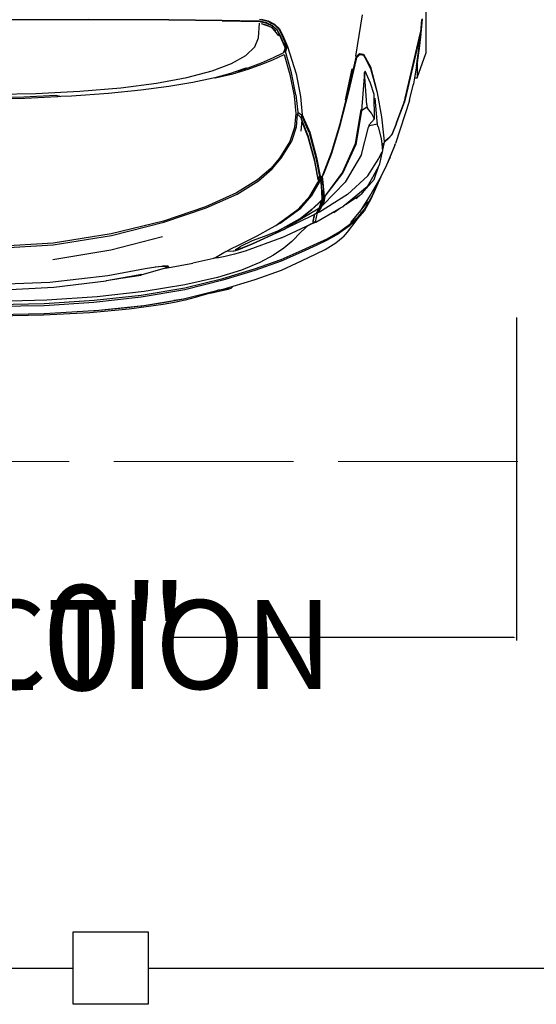
# Model space of a CAD drawing. Units: inches. Extents: x 0 to 4258, y 0 to 3769.
# Tile 7 of 30: x 3762 to 3797, y 2937 to 3003. Entities that reach past the tile are written whole.
import ezdxf

# ---------------------------------------------------------------- set-up
doc = ezdxf.new("R2010")
doc.units = ezdxf.units.IN
doc.header["$MEASUREMENT"] = 0
doc.linetypes.add('ACAD_ISO02W100', pattern=[15, 12, -3])
doc.layers.get('0').update_dxf_attribs({"color": 16})
for name, color, linetype, lineweight in [('A-ANNO-DIMS', 250, 'Continuous', 18), ('A-ANNO-TEXT', 250, 'Continuous', 18), ('A-FLOR-OVHD', 150, 'ACAD_ISO02W100', 13), ('C-PKNG-VEHI', 8, 'Continuous', 18), ('C-PROP', 150, 'Continuous', 25)]:
    doc.layers.add(name, color=color, linetype=linetype, lineweight=lineweight)
doc.layers.add('Edges', color=250, linetype='Continuous')
doc.styles.get("Standard").update_dxf_attribs({"font": 'arial.ttf'})
doc.dimstyles.get("Standard").update_dxf_attribs({"dimtxt": 7, "dimasz": 0.18, "dimexe": 0.18, "dimexo": 0.0625, "dimgap": 0.09, "dimtad": 0, "dimtih": 1, "dimtoh": 1, "dimzin": 0, "dimdsep": 46, "dimlunit": 3, "dimtxsty": 'Standard', "dimcen": 0.09, "dimadec": 0, "dimazin": 0, "dimtfac": 1, "dimtofl": 0, "dimtmove": 0, "dimatfit": 3, "dimfxl": 1, "dimtolj": 1, "dimtzin": 0, "dimarcsym": 0})

# ---------------------------------------------------------------- blocks, each defined once
blk = doc.blocks.new('Nissan Qashqai pl')
at = {"layer": 'Edges'}
for p, q in [((10.9577, 12.8101), (11.1283, 12.8101)), ((11.1783, 12.7921), (11.1283, 12.8101)), ((11.0576, 12.8026), (11.0798, 12.8008)), ((11.0768, 12.8008), (11.059, 12.8023)), ((11.0811, 12.8004), (11.0768, 12.8008)), ((11.0798, 12.8008), (11.0872, 12.7999)), ((11.0827, 12.8001), (11.0811, 12.8004)), ((11.0827, 12.8001), (11.0813, 12.7998)), ((11.0836, 12.8002), (11.0827, 12.8001)), ((11.0856, 12.7994), (11.0827, 12.8001)), ((11.0872, 12.7999), (11.0836, 12.8002)), ((11.0836, 12.8002), (11.0882, 12.7992)), ((11.2196, 12.7681), (11.0856, 12.7994)), ((11.0883, 12.7998), (11.0872, 12.7999)), ((11.0882, 12.7992), (11.2222, 12.7676)), ((11.0883, 12.7998), (11.1123, 12.797)), ((11.1147, 12.7965), (11.0883, 12.7998)), ((11.1123, 12.797), (11.1475, 12.7921)), ((11.1547, 12.791), (11.1147, 12.7965)), ((11.1475, 12.7921), (11.1525, 12.7914)), ((11.1475, 12.7921), (11.1783, 12.7921)), ((11.1525, 12.7914), (11.1547, 12.791)), ((11.1547, 12.791), (11.1783, 12.787)), ((11.1783, 12.787), (11.1783, 12.7921)), ((11.1783, 12.787), (11.1906, 12.7849)), ((11.1906, 12.7849), (11.1909, 12.7849)), ((11.193, 12.7845), (11.1909, 12.7849)), ((11.2215, 12.7775), (11.193, 12.7845)), ((11.2247, 12.7764), (11.2215, 12.7775)), ((11.2247, 12.7764), (11.3124, 12.7479)), ((11.2247, 12.767), (11.2163, 12.7689)), ((11.22, 12.768), (11.2196, 12.7681)), ((11.2247, 12.767), (11.22, 12.768)), ((11.2222, 12.7676), (11.2271, 12.7664)), ((11.2253, 12.7668), (11.2247, 12.767)), ((11.2304, 12.7649), (11.2253, 12.7668)), ((11.2253, 12.7668), (11.2271, 12.7664)), ((11.2271, 12.7664), (11.2296, 12.7658)), ((11.2271, 12.7664), (11.2277, 12.7662)), ((11.2277, 12.7662), (11.2296, 12.7658)), ((11.2732, 12.7496), (11.2277, 12.7662)), ((11.2704, 12.7504), (11.2304, 12.7649)), ((11.2702, 12.7507), (11.2704, 12.7504)), ((11.2704, 12.7506), (11.2707, 12.7503)), ((11.2707, 12.7503), (11.2704, 12.7504)), ((11.2719, 12.7498), (11.2707, 12.7503)), ((11.2934, 12.741), (11.2719, 12.7498)), ((11.2732, 12.7496), (11.2946, 12.7409)), ((11.3, 12.735), (11.2934, 12.741)), ((11.2946, 12.7409), (11.3018, 12.7346)), ((11.3081, 12.7253), (11.3, 12.735)), ((11.3018, 12.7346), (11.3103, 12.7249)), ((11.3161, 12.7467), (11.3124, 12.7479)), ((11.3161, 12.7467), (11.3376, 12.7381)), ((11.3192, 12.7454), (11.3566, 12.7294)), ((11.3405, 12.7369), (11.3376, 12.7381)), ((11.3405, 12.7369), (11.3566, 12.7294)), ((11.3566, 12.7294), (11.3796, 12.7187)), ((11.156, 12.6966), (11.203, 12.7093)), ((11.1589, 12.6971), (11.2062, 12.7098)), ((11.203, 12.7093), (11.2091, 12.7103)), ((11.2062, 12.7098), (11.2091, 12.7103)), ((11.2091, 12.7103), (11.2583, 12.7196)), ((11.2199, 12.706), (11.2666, 12.7097)), ((11.2583, 12.7196), (11.2956, 12.7234)), ((11.2666, 12.7097), (11.2729, 12.7104)), ((11.2787, 12.7123), (11.2729, 12.7104)), ((11.2729, 12.7104), (11.2766, 12.6957)), ((11.2787, 12.7123), (11.3022, 12.7186)), ((11.2956, 12.7234), (11.3085, 12.7247)), ((11.3022, 12.7186), (11.3252, 12.7213)), ((11.3086, 12.7247), (11.3081, 12.7253)), ((11.3081, 12.7253), (11.3087, 12.7247)), ((11.3085, 12.7247), (11.3086, 12.7247)), ((11.3086, 12.7247), (11.3087, 12.7247)), ((11.3087, 12.7247), (11.3103, 12.7249)), ((11.3103, 12.7249), (11.3103, 12.7249)), ((11.3103, 12.7249), (11.3106, 12.7249)), ((11.3106, 12.7249), (11.314, 12.7238)), ((11.317, 12.7227), (11.3119, 12.7236)), ((11.3132, 12.7243), (11.3256, 12.7215)), ((11.314, 12.7238), (11.317, 12.7227)), ((11.314, 12.7238), (11.3242, 12.7216)), ((11.3242, 12.7216), (11.317, 12.7227)), ((11.3198, 12.7211), (11.3252, 12.7213)), ((11.3242, 12.7216), (11.3256, 12.7215)), ((11.3252, 12.7213), (11.3283, 12.7214)), ((11.3256, 12.7215), (11.3283, 12.7214)), ((11.3283, 12.7214), (11.3297, 12.7206)), ((11.3297, 12.7206), (11.3446, 12.7173)), ((11.3297, 12.7206), (11.3302, 12.7203)), ((11.3302, 12.7203), (11.3446, 12.7173)), ((11.3302, 12.7203), (11.3394, 12.7152)), ((11.3394, 12.7152), (11.3434, 12.7138)), ((11.3394, 12.7152), (11.342, 12.7137)), ((11.379, 12.6915), (11.3434, 12.7138)), ((11.3446, 12.7173), (11.3571, 12.7146)), ((11.3583, 12.7142), (11.3571, 12.7146)), ((11.3571, 12.7146), (11.3821, 12.7008)), ((11.3583, 12.7142), (11.3821, 12.7008)), ((11.3864, 12.7044), (11.3583, 12.7142)), ((11.3796, 12.7187), (11.4164, 12.6974)), ((11.3796, 12.7187), (11.3807, 12.7182)), ((11.3807, 12.7182), (11.4267, 12.6979)), ((11.4228, 12.6989), (11.3807, 12.7182)), ((11.1298, 12.6823), (11.156, 12.6966)), ((11.1365, 12.6851), (11.1589, 12.6971)), ((11.189, 12.6968), (11.1644, 12.6862)), ((11.2337, 12.6892), (11.1672, 12.6844)), ((11.2121, 12.7043), (11.189, 12.6968)), ((11.2622, 12.7051), (11.2121, 12.7043)), ((11.2337, 12.6892), (11.2382, 12.6892)), ((11.2382, 12.6892), (11.2401, 12.6908)), ((11.2382, 12.6892), (11.2459, 12.6785)), ((11.2505, 12.6987), (11.2401, 12.6908)), ((11.2601, 12.7037), (11.2505, 12.6987)), ((11.2622, 12.7051), (11.2601, 12.7037)), ((11.2743, 12.6942), (11.2622, 12.7051)), ((11.2743, 12.6942), (11.2791, 12.6927)), ((11.335, 12.6786), (11.2791, 12.6927)), ((11.379, 12.6915), (11.417, 12.6499)), ((11.3821, 12.7008), (11.4014, 12.69)), ((11.4163, 12.6775), (11.3864, 12.7044)), ((11.4014, 12.69), (11.4022, 12.6894)), ((11.4014, 12.69), (11.4265, 12.6594)), ((11.4022, 12.6894), (11.4163, 12.6775)), ((11.4022, 12.6894), (11.4265, 12.6594)), ((11.4164, 12.6974), (11.4531, 12.6744)), ((11.4243, 12.6982), (11.4228, 12.6989)), ((11.4464, 12.6853), (11.4243, 12.6982)), ((11.4267, 12.6979), (11.4498, 12.6844)), ((11.4531, 12.6744), (11.4314, 12.6911)), ((11.1336, 12.667), (11.0492, 12.6807)), ((11.1285, 12.6745), (11.1298, 12.6823)), ((11.1293, 12.6736), (11.1285, 12.6745)), ((11.1306, 12.6812), (11.1293, 12.6736)), ((11.1353, 12.6677), (11.1293, 12.6736)), ((11.1306, 12.6752), (11.1319, 12.6827)), ((11.1319, 12.6827), (11.1306, 12.6812)), ((11.1347, 12.671), (11.1306, 12.6752)), ((11.1319, 12.6827), (11.1365, 12.6851)), ((11.1366, 12.6691), (11.1347, 12.671)), ((11.1358, 12.6676), (11.1366, 12.6691)), ((11.1401, 12.6682), (11.1366, 12.6691)), ((11.1644, 12.6862), (11.1672, 12.6844)), ((11.1672, 12.6844), (11.2459, 12.6785)), ((11.2428, 12.6769), (11.3132, 12.6652)), ((11.2459, 12.6785), (11.3153, 12.6672)), ((11.335, 12.6786), (11.3915, 12.6453)), ((11.4366, 12.6471), (11.4163, 12.6775)), ((11.4163, 12.6775), (11.4259, 12.6674)), ((11.4624, 12.6717), (11.4464, 12.6853)), ((11.4498, 12.6844), (11.4662, 12.6706)), ((11.4681, 12.6691), (11.4498, 12.6844)), ((11.4742, 12.6567), (11.4531, 12.6744)), ((11.4774, 12.6543), (11.4624, 12.6717)), ((11.4662, 12.6706), (11.4815, 12.6531)), ((11.4681, 12.6691), (11.4936, 12.6491)), ((11.1358, 12.6676), (11.1353, 12.6677)), ((11.148, 12.665), (11.1358, 12.6676)), ((11.2066, 12.6527), (11.1401, 12.6682)), ((11.2063, 12.6515), (11.148, 12.665)), ((11.2232, 12.6458), (11.1598, 12.6594)), ((11.272, 12.6349), (11.2063, 12.6515)), ((11.2728, 12.6357), (11.2066, 12.6527)), ((11.3132, 12.6652), (11.3715, 12.6398)), ((11.3733, 12.6404), (11.3153, 12.6672)), ((11.417, 12.6499), (11.4529, 12.5922)), ((11.4265, 12.6594), (11.4366, 12.6471)), ((11.4924, 12.6339), (11.4774, 12.6543)), ((11.4815, 12.6531), (11.4963, 12.6328)), ((11.4936, 12.6491), (11.5033, 12.6408)), ((11.3311, 12.6172), (11.272, 12.6349)), ((11.3323, 12.6178), (11.2728, 12.6357)), ((11.3715, 12.6398), (11.4177, 12.6052)), ((11.4203, 12.6044), (11.3733, 12.6404)), ((11.3915, 12.6453), (11.4381, 12.6002)), ((11.4366, 12.6471), (11.4408, 12.6419)), ((11.4408, 12.6419), (11.4411, 12.6414)), ((11.4411, 12.6414), (11.4411, 12.6414)), ((11.4414, 12.6409), (11.4411, 12.6414)), ((11.4414, 12.6409), (11.447, 12.6315)), ((11.4455, 12.6336), (11.4414, 12.6409)), ((11.447, 12.6315), (11.4455, 12.6336)), ((11.4455, 12.6336), (11.4462, 12.6324)), ((11.447, 12.6315), (11.4462, 12.6324)), ((11.4732, 12.585), (11.4462, 12.6324)), ((11.447, 12.6315), (11.447, 12.6314)), ((11.4536, 12.6215), (11.447, 12.6314)), ((11.5074, 12.608), (11.4924, 12.6339)), ((11.4964, 12.6326), (11.4963, 12.6328)), ((11.4964, 12.6326), (11.5113, 12.6069)), ((11.5158, 12.6256), (11.5033, 12.6408)), ((11.3751, 12.5999), (11.3311, 12.6172)), ((11.3747, 12.6011), (11.3323, 12.6178)), ((11.5165, 12.5882), (11.5074, 12.608)), ((11.5295, 12.6041), (11.5158, 12.6256)), ((11.3411, 12.5863), (11.3795, 12.5939)), ((11.3419, 12.585), (11.3804, 12.5926)), ((11.3847, 12.5899), (11.3474, 12.5827)), ((11.3863, 12.5898), (11.3493, 12.5828)), ((11.38, 12.5988), (11.3747, 12.6011)), ((11.3751, 12.5999), (11.3762, 12.5999)), ((11.3752, 12.5998), (11.3751, 12.5999)), ((11.3763, 12.5998), (11.3752, 12.5998)), ((11.3764, 12.5993), (11.3752, 12.5998)), ((11.3792, 12.5982), (11.3764, 12.5993)), ((11.3792, 12.5982), (11.3793, 12.5979)), ((11.3792, 12.5982), (11.3804, 12.5972)), ((11.3795, 12.5939), (11.3834, 12.5947)), ((11.3853, 12.5993), (11.38, 12.5988)), ((11.3804, 12.5972), (11.4082, 12.5998)), ((11.3827, 12.5953), (11.3804, 12.5972)), ((11.3804, 12.5926), (11.3841, 12.5933)), ((11.3847, 12.5899), (11.3804, 12.5926)), ((11.3811, 12.5958), (11.3808, 12.5961)), ((11.3834, 12.5947), (11.3827, 12.5953)), ((11.3846, 12.5953), (11.3829, 12.5952)), ((11.3829, 12.5952), (11.3849, 12.5951)), ((11.388, 12.591), (11.3829, 12.5952)), ((11.3834, 12.5947), (11.3841, 12.5933)), ((11.3846, 12.5953), (11.4248, 12.5976)), ((11.3846, 12.5953), (11.3846, 12.5953)), ((11.3851, 12.5951), (11.3846, 12.5953)), ((11.3846, 12.5953), (11.3849, 12.5951)), ((11.3847, 12.5899), (11.3848, 12.5899)), ((11.388, 12.591), (11.3848, 12.5899)), ((11.3849, 12.5951), (11.3851, 12.5951)), ((11.3882, 12.5923), (11.3849, 12.5951)), ((11.3851, 12.5951), (11.3867, 12.5949)), ((11.4171, 12.5766), (11.3851, 12.5951)), ((11.4212, 12.603), (11.3853, 12.5993)), ((11.3895, 12.5912), (11.3863, 12.5898)), ((11.3867, 12.5949), (11.3915, 12.5951)), ((11.3914, 12.5926), (11.3867, 12.5949)), ((11.3886, 12.5919), (11.3872, 12.5927)), ((11.3882, 12.5923), (11.3886, 12.5919)), ((11.3886, 12.5919), (11.3895, 12.5912)), ((11.3892, 12.5916), (11.3886, 12.5919)), ((11.3923, 12.5894), (11.3895, 12.5912)), ((11.4187, 12.5768), (11.3914, 12.5926)), ((11.3915, 12.5951), (11.4266, 12.5977)), ((11.4203, 12.5724), (11.3923, 12.5894)), ((11.409, 12.5999), (11.4082, 12.5998)), ((11.4164, 12.5998), (11.4082, 12.5998)), ((11.4152, 12.6004), (11.409, 12.5999)), ((11.409, 12.5999), (11.4163, 12.5999)), ((11.4173, 12.6006), (11.4152, 12.6004)), ((11.4163, 12.5999), (11.4152, 12.6004)), ((11.4163, 12.5999), (11.4186, 12.5999)), ((11.4164, 12.5998), (11.4163, 12.5999)), ((11.4181, 12.5998), (11.4164, 12.5998)), ((11.4169, 12.5996), (11.4164, 12.5998)), ((11.4252, 12.598), (11.4169, 12.5996)), ((11.4176, 12.6007), (11.4173, 12.6006)), ((11.418, 12.6006), (11.4173, 12.6006)), ((11.4215, 12.601), (11.4176, 12.6007)), ((11.418, 12.6006), (11.4176, 12.6007)), ((11.4177, 12.6052), (11.4193, 12.6042)), ((11.4204, 12.6002), (11.418, 12.6006)), ((11.4194, 12.6), (11.418, 12.6006)), ((11.4192, 12.6045), (11.4194, 12.6042)), ((11.4194, 12.6042), (11.4193, 12.6042)), ((11.4193, 12.6042), (11.4196, 12.604)), ((11.4194, 12.6042), (11.4196, 12.604)), ((11.4196, 12.6042), (11.4194, 12.6042)), ((11.4196, 12.604), (11.4201, 12.6036)), ((11.4198, 12.6041), (11.4201, 12.6036)), ((11.4201, 12.6036), (11.4212, 12.603)), ((11.4292, 12.6024), (11.4203, 12.6044)), ((11.4229, 12.6025), (11.4203, 12.6044)), ((11.4212, 12.603), (11.4215, 12.601)), ((11.4218, 12.6028), (11.4212, 12.603)), ((11.4215, 12.601), (11.4219, 12.6009)), ((11.4222, 12.6029), (11.4218, 12.6028)), ((11.4229, 12.6025), (11.4218, 12.6028)), ((11.4219, 12.6009), (11.4222, 12.6005)), ((11.4219, 12.6009), (11.4224, 12.6008)), ((11.4224, 12.6008), (11.4226, 12.6006)), ((11.4224, 12.6008), (11.423, 12.6006)), ((11.4315, 12.6002), (11.4229, 12.6025)), ((11.423, 12.6006), (11.4229, 12.6025)), ((11.44, 12.5959), (11.423, 12.6006)), ((11.4248, 12.5976), (11.4266, 12.5977)), ((11.4266, 12.5977), (11.4252, 12.598)), ((11.4266, 12.5977), (11.4268, 12.5977)), ((11.4268, 12.5977), (11.4296, 12.5954)), ((11.4268, 12.5977), (11.4278, 12.5977)), ((11.4303, 12.5956), (11.4278, 12.5977)), ((11.4278, 12.5977), (11.43, 12.5969)), ((11.4381, 12.6002), (11.4292, 12.6024)), ((11.4296, 12.5954), (11.4469, 12.5773)), ((11.4337, 12.5962), (11.43, 12.5969)), ((11.43, 12.5969), (11.4361, 12.5948)), ((11.4479, 12.5766), (11.4303, 12.5956)), ((11.4403, 12.5978), (11.4315, 12.6002)), ((11.4397, 12.5937), (11.4337, 12.5962)), ((11.4361, 12.5948), (11.4406, 12.5932)), ((11.4381, 12.6002), (11.4403, 12.5978)), ((11.4406, 12.5932), (11.4397, 12.5937)), ((11.4403, 12.5978), (11.44, 12.5959)), ((11.44, 12.5959), (11.4457, 12.5928)), ((11.4462, 12.5947), (11.4403, 12.5978)), ((11.4406, 12.5932), (11.4442, 12.592)), ((11.4442, 12.592), (11.4497, 12.589)), ((11.4462, 12.5893), (11.4442, 12.592)), ((11.4457, 12.5928), (11.4512, 12.5893)), ((11.452, 12.591), (11.4462, 12.5947)), ((11.475, 12.5409), (11.4462, 12.5893)), ((11.4497, 12.589), (11.4498, 12.5889)), ((11.4535, 12.5876), (11.4498, 12.5889)), ((11.4498, 12.5889), (11.4549, 12.5855)), ((11.4512, 12.5893), (11.4535, 12.5876)), ((11.4539, 12.5897), (11.452, 12.591)), ((11.4529, 12.5922), (11.4542, 12.5894)), ((11.4535, 12.5876), (11.4532, 12.5882)), ((11.4535, 12.5876), (11.4542, 12.5894)), ((11.4542, 12.5894), (11.4539, 12.5897)), ((11.5113, 12.6068), (11.5113, 12.6069)), ((11.5113, 12.6068), (11.5206, 12.5869)), ((11.5306, 12.5573), (11.5165, 12.5882)), ((11.5384, 12.5859), (11.5295, 12.6041)), ((11.29, 12.5711), (11.2541, 12.5557)), ((11.2586, 12.5591), (11.2895, 12.5724)), ((11.2972, 12.5692), (11.2677, 12.5575)), ((11.2993, 12.5695), (11.2705, 12.5579)), ((11.2895, 12.5724), (11.3411, 12.5863)), ((11.29, 12.5711), (11.3419, 12.585)), ((11.3474, 12.5827), (11.2972, 12.5692)), ((11.3493, 12.5828), (11.2993, 12.5695)), ((11.3474, 12.5827), (11.3474, 12.5827)), ((11.4433, 12.5543), (11.4171, 12.5766)), ((11.4447, 12.5545), (11.4187, 12.5768)), ((11.4467, 12.5488), (11.4203, 12.5724)), ((11.4469, 12.5773), (11.4659, 12.5539)), ((11.4654, 12.5548), (11.4479, 12.5766)), ((11.4535, 12.5876), (11.4728, 12.5838)), ((11.4549, 12.5855), (11.4568, 12.5836)), ((11.4564, 12.5833), (11.4567, 12.5833)), ((11.4569, 12.583), (11.4565, 12.5831)), ((11.4568, 12.5836), (11.4571, 12.5833)), ((11.4571, 12.5833), (11.4573, 12.583)), ((11.4573, 12.583), (11.4578, 12.5822)), ((11.4704, 12.5803), (11.4573, 12.583)), ((11.4573, 12.5823), (11.4574, 12.5822)), ((11.4573, 12.5823), (11.4573, 12.5823)), ((11.4576, 12.5822), (11.4574, 12.5822)), ((11.4578, 12.5822), (11.4588, 12.5807)), ((11.4605, 12.5816), (11.4578, 12.5822)), ((11.4588, 12.5807), (11.4895, 12.5178)), ((11.4713, 12.5794), (11.4605, 12.5816)), ((11.4742, 12.5797), (11.4704, 12.5803)), ((11.4744, 12.5792), (11.4713, 12.5794)), ((11.4732, 12.585), (11.4728, 12.5838)), ((11.4728, 12.5838), (11.4742, 12.5797)), ((11.4728, 12.5838), (11.4746, 12.5796)), ((11.4758, 12.5791), (11.4732, 12.585)), ((11.4742, 12.5797), (11.4744, 12.5792)), ((11.4745, 12.5797), (11.4742, 12.5797)), ((11.4745, 12.5792), (11.4744, 12.5792)), ((11.4745, 12.5792), (11.4745, 12.5797)), ((11.4745, 12.5797), (11.4746, 12.5796)), ((11.4748, 12.5792), (11.4745, 12.5792)), ((11.4746, 12.5796), (11.4748, 12.5792)), ((11.4746, 12.5796), (11.4758, 12.5791)), ((11.4758, 12.5791), (11.4748, 12.5792)), ((11.4758, 12.5791), (11.4759, 12.579)), ((11.4759, 12.579), (11.4778, 12.5746)), ((11.4759, 12.579), (11.4771, 12.576)), ((11.5057, 12.5145), (11.4771, 12.576)), ((11.4778, 12.5746), (11.4826, 12.5669)), ((11.5206, 12.5869), (11.5349, 12.5559)), ((11.5527, 12.5559), (11.5384, 12.5859)), ((11.1702, 12.5444), (11.2166, 12.5534)), ((11.2127, 12.5443), (11.2488, 12.548)), ((11.2166, 12.5534), (11.2538, 12.5571)), ((11.2488, 12.548), (11.2541, 12.5557)), ((11.2488, 12.548), (11.2524, 12.5477)), ((11.2599, 12.5552), (11.2524, 12.5477)), ((11.2785, 12.5455), (11.2524, 12.5477)), ((11.2538, 12.5571), (11.2586, 12.5591)), ((11.2541, 12.5557), (11.2599, 12.5552)), ((11.2677, 12.5575), (11.2599, 12.5552)), ((11.265, 12.5563), (11.2599, 12.5552)), ((11.2705, 12.5579), (11.265, 12.5563)), ((11.265, 12.5563), (11.2724, 12.5557)), ((11.2724, 12.5557), (11.2874, 12.5544)), ((11.4745, 12.5116), (11.4433, 12.5543)), ((11.4758, 12.5118), (11.4447, 12.5545)), ((11.4801, 12.503), (11.4467, 12.5488)), ((11.4633, 12.5594), (11.4897, 12.5108)), ((11.4654, 12.5548), (11.4659, 12.5539)), ((11.4659, 12.5539), (11.4674, 12.5512)), ((11.4675, 12.551), (11.4674, 12.5512)), ((11.4675, 12.551), (11.4703, 12.546)), ((11.4826, 12.5669), (11.4869, 12.5615)), ((11.4869, 12.5615), (11.4933, 12.555)), ((11.5131, 12.5356), (11.4933, 12.555)), ((11.5496, 12.5141), (11.5306, 12.5573)), ((11.5349, 12.5559), (11.5535, 12.5139)), ((11.5716, 12.5145), (11.5527, 12.5559)), ((11.1144, 12.5271), (11.1702, 12.5444)), ((11.1683, 12.5354), (11.1244, 12.5227)), ((11.1302, 12.52), (11.1712, 12.5317)), ((11.2127, 12.5443), (11.1683, 12.5354)), ((11.1712, 12.5317), (11.2152, 12.5404)), ((11.2152, 12.5404), (11.2509, 12.5439)), ((11.2509, 12.5439), (11.28, 12.5414)), ((11.3076, 12.5358), (11.2785, 12.5455)), ((11.28, 12.5414), (11.3082, 12.532)), ((11.3428, 12.5139), (11.3076, 12.5358)), ((11.3082, 12.532), (11.3425, 12.5106)), ((11.4703, 12.546), (11.4704, 12.5458)), ((11.4704, 12.5458), (11.4909, 12.5085)), ((11.4704, 12.5458), (11.4897, 12.5108)), ((11.475, 12.5409), (11.4828, 12.5276)), ((11.488, 12.5208), (11.4828, 12.5276)), ((11.5131, 12.5356), (11.5265, 12.5194)), ((11.0682, 12.5004), (11.0779, 12.5103)), ((11.0692, 12.4996), (11.0787, 12.5092)), ((11.0747, 12.4944), (11.092, 12.5087)), ((11.0779, 12.5103), (11.0902, 12.5166)), ((11.0787, 12.5092), (11.0908, 12.5153)), ((11.0912, 12.5117), (11.0802, 12.5057)), ((11.0917, 12.5114), (11.0809, 12.5056)), ((11.0902, 12.5166), (11.1144, 12.5271)), ((11.0908, 12.5153), (11.107, 12.5224)), ((11.1138, 12.5213), (11.0912, 12.5117)), ((11.1149, 12.5212), (11.0917, 12.5114)), ((11.107, 12.5224), (11.1116, 12.5243)), ((11.1138, 12.5213), (11.107, 12.5224)), ((11.1116, 12.5243), (11.1147, 12.5257)), ((11.1244, 12.5227), (11.1116, 12.5243)), ((11.1139, 12.5213), (11.1138, 12.5213)), ((11.1164, 12.5224), (11.1139, 12.5213)), ((11.1147, 12.5257), (11.1244, 12.5227)), ((11.1172, 12.5222), (11.1149, 12.5212)), ((11.1164, 12.5224), (11.1174, 12.5223)), ((11.1173, 12.5222), (11.1172, 12.5222)), ((11.1174, 12.5223), (11.1173, 12.5222)), ((11.12, 12.5215), (11.1174, 12.5223)), ((11.1246, 12.5199), (11.12, 12.5215)), ((11.1259, 12.5194), (11.1244, 12.5227)), ((11.1244, 12.5227), (11.126, 12.5194)), ((11.1259, 12.5194), (11.1246, 12.5199)), ((11.126, 12.5193), (11.1247, 12.5197)), ((11.126, 12.5193), (11.1248, 12.5195)), ((11.1251, 12.5189), (11.126, 12.5193)), ((11.126, 12.5193), (11.1259, 12.5194)), ((11.126, 12.5194), (11.1259, 12.5194)), ((11.126, 12.5194), (11.1261, 12.5193)), ((11.1264, 12.5192), (11.126, 12.5194)), ((11.1263, 12.5186), (11.126, 12.5193)), ((11.1261, 12.5193), (11.126, 12.5193)), ((11.1261, 12.5193), (11.1263, 12.5188)), ((11.1264, 12.5192), (11.1261, 12.5193)), ((11.1277, 12.5167), (11.1264, 12.5192)), ((11.1369, 12.4986), (11.1277, 12.5167)), ((11.1412, 12.4969), (11.1302, 12.52)), ((11.3425, 12.5106), (11.3635, 12.4929)), ((11.3645, 12.4958), (11.3428, 12.5139)), ((11.4788, 12.5052), (11.4745, 12.5116)), ((11.4852, 12.494), (11.4758, 12.5118)), ((11.5179, 12.4551), (11.488, 12.5208)), ((11.4898, 12.5172), (11.4895, 12.5178)), ((11.4897, 12.5108), (11.4909, 12.5085)), ((11.4898, 12.5172), (11.49, 12.5167)), ((11.49, 12.5167), (11.5179, 12.4551)), ((11.4909, 12.5085), (11.5028, 12.4792)), ((11.5057, 12.5145), (11.5325, 12.4404)), ((11.5265, 12.5194), (11.541, 12.4982)), ((11.5691, 12.4592), (11.5496, 12.5141)), ((11.5535, 12.5139), (11.5726, 12.46)), ((11.5908, 12.4606), (11.5716, 12.5145)), ((11.0581, 12.4738), (11.0614, 12.4872)), ((11.0614, 12.4872), (11.0682, 12.5004)), ((11.0624, 12.4866), (11.0658, 12.4932)), ((11.0658, 12.4932), (11.0692, 12.4996)), ((11.0658, 12.4932), (11.0698, 12.4925)), ((11.0698, 12.4925), (11.0659, 12.4848)), ((11.0727, 12.4966), (11.0669, 12.4849)), ((11.0671, 12.4731), (11.0747, 12.4944)), ((11.0696, 12.4836), (11.0747, 12.4944)), ((11.0718, 12.4967), (11.0698, 12.4925)), ((11.0802, 12.5057), (11.0718, 12.4967)), ((11.0809, 12.5056), (11.0727, 12.4966)), ((11.0747, 12.4944), (11.0821, 12.5029)), ((11.1475, 12.4741), (11.1369, 12.4986)), ((11.1505, 12.4742), (11.1412, 12.4969)), ((11.3635, 12.4929), (11.3872, 12.4654)), ((11.3888, 12.4678), (11.3645, 12.4958)), ((11.4801, 12.503), (11.4788, 12.5052)), ((11.4852, 12.494), (11.4801, 12.503)), ((11.5013, 12.4651), (11.4852, 12.494)), ((11.541, 12.4982), (11.5562, 12.4701)), ((11.0582, 12.47), (11.0624, 12.4866)), ((11.0618, 12.3933), (11.0632, 12.47)), ((11.0622, 12.4697), (11.0621, 12.4657)), ((11.063, 12.4728), (11.0622, 12.4697)), ((11.0659, 12.4848), (11.063, 12.4728)), ((11.0641, 12.4733), (11.0632, 12.47)), ((11.0669, 12.4849), (11.0641, 12.4733)), ((11.0962, 12.4675), (11.0662, 12.4698)), ((11.0671, 12.4731), (11.0696, 12.4836)), ((11.1148, 12.4598), (11.0962, 12.4675)), ((11.1577, 12.4465), (11.1475, 12.4741)), ((11.1605, 12.4465), (11.1505, 12.4742)), ((11.4159, 12.4242), (11.3888, 12.4678)), ((11.5028, 12.4792), (11.5118, 12.4548)), ((11.5562, 12.4701), (11.5715, 12.4326)), ((11.0621, 12.4657), (11.0607, 12.3933)), ((11.1323, 12.4415), (11.1148, 12.4598)), ((11.3872, 12.4654), (11.4138, 12.4223)), ((11.5202, 12.427), (11.5013, 12.4651)), ((11.5118, 12.4548), (11.523, 12.4311)), ((11.5118, 12.4548), (11.513, 12.4514)), ((11.5292, 12.4272), (11.5179, 12.4551)), ((11.5179, 12.4551), (11.5285, 12.4279)), ((11.5884, 12.3943), (11.5691, 12.4592)), ((11.5726, 12.46), (11.5922, 12.3947)), ((11.6042, 12.4156), (11.5908, 12.4606)), ((11.1487, 12.4126), (11.1323, 12.4415)), ((11.1643, 12.425), (11.1576, 12.4459)), ((11.1643, 12.425), (11.1577, 12.4465)), ((11.1582, 12.4416), (11.1668, 12.4177)), ((11.1583, 12.4423), (11.1643, 12.425)), ((11.1699, 12.4153), (11.1605, 12.4465)), ((11.5283, 12.4109), (11.5202, 12.427)), ((11.5301, 12.4198), (11.523, 12.4311)), ((11.5285, 12.4279), (11.5302, 12.4209)), ((11.5331, 12.4157), (11.5292, 12.4272)), ((11.5325, 12.4404), (11.5386, 12.4187)), ((11.5715, 12.4326), (11.5866, 12.3835)), ((11.164, 12.373), (11.1487, 12.4126)), ((11.1643, 12.425), (11.1668, 12.4177)), ((11.1668, 12.4177), (11.1694, 12.4104)), ((11.1694, 12.4104), (11.1781, 12.3782)), ((11.178, 12.379), (11.1699, 12.4153)), ((11.4138, 12.4223), (11.4422, 12.3594)), ((11.4445, 12.3608), (11.4159, 12.4242)), ((11.5334, 12.4014), (11.5283, 12.4109)), ((11.5302, 12.4209), (11.5301, 12.4198)), ((11.5331, 12.4157), (11.5335, 12.401)), ((11.5386, 12.4187), (11.5434, 12.3997)), ((11.6042, 12.4156), (11.6077, 12.4125)), ((11.6103, 12.395), (11.6042, 12.4156)), ((11.6077, 12.4125), (11.6094, 12.4107)), ((11.6094, 12.4107), (11.6101, 12.4085)), ((11.6101, 12.4085), (11.6127, 12.3852)), ((11.6185, 12.3689), (11.6101, 12.4085)), ((11.0607, 12.3933), (11.0595, 12.2842)), ((11.0618, 12.3933), (11.0606, 12.2841)), ((11.5326, 12.4045), (11.5333, 12.4019)), ((11.5333, 12.4019), (11.5334, 12.4014)), ((11.5335, 12.401), (11.5334, 12.4014)), ((11.5357, 12.3968), (11.5335, 12.401)), ((11.5416, 12.3863), (11.5357, 12.3968)), ((11.5434, 12.3997), (11.5461, 12.3854)), ((11.6076, 12.3166), (11.5884, 12.3943)), ((11.5922, 12.3947), (11.6118, 12.3165)), ((11.6127, 12.3852), (11.6103, 12.395)), ((11.1776, 12.3211), (11.164, 12.373)), ((11.1781, 12.3782), (11.178, 12.379)), ((11.1781, 12.3782), (11.1791, 12.3746)), ((11.1791, 12.3746), (11.1877, 12.333)), ((11.5455, 12.3793), (11.5416, 12.3863)), ((11.5472, 12.3757), (11.5455, 12.3793)), ((11.5461, 12.3854), (11.5467, 12.3822)), ((11.5467, 12.3822), (11.5571, 12.3331)), ((11.5866, 12.3835), (11.6016, 12.3166)), ((11.6127, 12.3852), (11.6174, 12.3722)), ((11.6297, 12.3166), (11.6127, 12.3852)), ((11.6174, 12.3722), (11.6185, 12.3689)), ((11.6185, 12.3689), (11.6224, 12.3567)), ((11.4422, 12.3594), (11.4712, 12.2729)), ((11.4738, 12.274), (11.4445, 12.3608)), ((11.6224, 12.3567), (11.6277, 12.3379)), ((11.1877, 12.333), (11.1958, 12.2844)), ((11.5668, 12.2816), (11.5571, 12.3331)), ((11.6277, 12.3379), (11.6328, 12.3174)), ((11.1891, 12.2586), (11.1776, 12.3211)), ((11.6016, 12.3166), (11.615, 12.2333)), ((11.6229, 12.2274), (11.6076, 12.3166)), ((11.6118, 12.3165), (11.6272, 12.2272)), ((11.6301, 12.3141), (11.6297, 12.3166)), ((11.6377, 12.2734), (11.6301, 12.3141)), ((11.6332, 12.2951), (11.6301, 12.3141)), ((11.6328, 12.3174), (11.6375, 12.2956)), ((11.6334, 12.2946), (11.6332, 12.2951)), ((11.6443, 12.2288), (11.6334, 12.2946)), ((11.6375, 12.2956), (11.6422, 12.2725)), ((11.0595, 12.2842), (11.0586, 12.1198)), ((11.0606, 12.2841), (11.0597, 12.1196)), ((11.1958, 12.2844), (11.2033, 12.2269)), ((11.4712, 12.2729), (11.4976, 12.1662)), ((11.5005, 12.167), (11.4738, 12.274)), ((11.5033, 12.271), (11.5307, 12.165)), ((11.5626, 12.2771), (11.5627, 12.2817)), ((11.5627, 12.2746), (11.5626, 12.2771)), ((11.5626, 12.2745), (11.5627, 12.2746)), ((11.5627, 12.2817), (11.5634, 12.2829)), ((11.5627, 12.2817), (11.5633, 12.2814)), ((11.5628, 12.2721), (11.5627, 12.2746)), ((11.5632, 12.2783), (11.5633, 12.2814)), ((11.5636, 12.2706), (11.5632, 12.2783)), ((11.5633, 12.2814), (11.5634, 12.2829)), ((11.5633, 12.2814), (11.5661, 12.2803)), ((11.5634, 12.2829), (11.5668, 12.2816)), ((11.565, 12.2577), (11.5636, 12.2706)), ((11.5639, 12.2809), (11.5637, 12.2764)), ((11.5637, 12.2763), (11.5637, 12.2764)), ((11.5637, 12.2764), (11.5638, 12.2762)), ((11.5638, 12.2762), (11.5641, 12.2688)), ((11.5643, 12.2808), (11.5639, 12.2809)), ((11.5641, 12.2688), (11.5656, 12.2559)), ((11.5642, 12.2771), (11.5646, 12.2778)), ((11.566, 12.2801), (11.5643, 12.2808)), ((11.5647, 12.278), (11.5649, 12.2783)), ((11.566, 12.2846), (11.5668, 12.2816)), ((11.566, 12.2801), (11.5661, 12.2803)), ((11.5662, 12.28), (11.566, 12.2801)), ((11.5661, 12.2803), (11.5662, 12.28)), ((11.5662, 12.28), (11.5661, 12.2803)), ((11.5669, 12.2797), (11.5661, 12.2803)), ((11.5669, 12.2797), (11.5662, 12.28)), ((11.5662, 12.28), (11.5662, 12.28)), ((11.5667, 12.2813), (11.567, 12.2796)), ((11.5668, 12.2816), (11.5672, 12.2796)), ((11.567, 12.2796), (11.5669, 12.2797)), ((11.5672, 12.2796), (11.567, 12.2796)), ((11.5678, 12.2766), (11.5672, 12.2796)), ((11.5673, 12.2784), (11.5677, 12.2767)), ((11.5678, 12.2766), (11.5818, 12.227)), ((11.5682, 12.2743), (11.5682, 12.2742)), ((11.5683, 12.2739), (11.5683, 12.2739)), ((11.5683, 12.2738), (11.5683, 12.2737)), ((11.6378, 12.2728), (11.6377, 12.2734)), ((11.6381, 12.2716), (11.6378, 12.2728)), ((11.639, 12.2645), (11.6378, 12.2728)), ((11.639, 12.2645), (11.6381, 12.2716)), ((11.6422, 12.2725), (11.6514, 12.2026)), ((11.1984, 12.1855), (11.1891, 12.2586)), ((11.5685, 12.2359), (11.565, 12.2577)), ((11.6443, 12.2288), (11.639, 12.2645)), ((11.2033, 12.2269), (11.21, 12.1607)), ((11.5823, 12.1589), (11.5685, 12.2359)), ((11.593, 12.1566), (11.58, 12.2288)), ((11.5883, 12.186), (11.5816, 12.2272)), ((11.5883, 12.186), (11.5818, 12.227)), ((11.615, 12.2333), (11.626, 12.1375)), ((11.6333, 12.131), (11.6229, 12.2274)), ((11.6272, 12.2272), (11.6377, 12.1308)), ((11.6446, 12.2271), (11.6443, 12.2288)), ((11.6448, 12.2258), (11.6446, 12.2271)), ((11.6474, 12.2042), (11.6448, 12.2258)), ((11.6539, 12.1338), (11.6448, 12.2258)), ((11.2057, 12.1019), (11.1984, 12.1855)), ((11.593, 12.1566), (11.5883, 12.186)), ((11.6474, 12.2038), (11.6474, 12.2042)), ((11.6475, 12.2032), (11.6474, 12.2038)), ((11.648, 12.198), (11.6475, 12.2032)), ((11.6539, 12.1338), (11.648, 12.198)), ((11.6514, 12.2026), (11.6589, 12.1222)), ((11.4976, 12.1662), (11.5166, 12.0471)), ((11.5196, 12.0475), (11.5005, 12.167)), ((11.5307, 12.165), (11.5504, 12.0466)), ((11.21, 12.1607), (11.2159, 12.085)), ((11.5963, 12.0406), (11.5823, 12.1589)), ((11.5932, 12.1556), (11.593, 12.1566)), ((11.6067, 12.0489), (11.5932, 12.1556)), ((11.626, 12.1375), (11.6329, 12.0344)), ((11.6399, 12.029), (11.6333, 12.131)), ((11.6377, 12.1308), (11.6444, 12.0289)), ((11.6543, 12.1306), (11.6539, 12.1338)), ((11.6604, 12.0287), (11.6543, 12.1306)), ((11.0597, 12.1196), (11.0594, 11.9221)), ((11.6589, 12.1222), (11.6635, 12.0274)), ((11.2101, 12.012), (11.2057, 12.1019)), ((11.2159, 12.085), (11.2166, 12.063)), ((11.2139, 12.0528), (11.2158, 12.0599)), ((11.2174, 11.9874), (11.2139, 12.0528)), ((11.2158, 12.0602), (11.2166, 12.063)), ((11.2158, 12.0602), (11.2168, 12.056)), ((11.2158, 12.0599), (11.2158, 12.0602)), ((11.2158, 12.0599), (11.2168, 12.056)), ((11.2168, 12.056), (11.2204, 11.989)), ((11.5166, 12.0471), (11.5239, 11.9221)), ((11.527, 11.9221), (11.5196, 12.0475)), ((11.6133, 11.9221), (11.6067, 12.0489)), ((11.6005, 11.9335), (11.5963, 12.0406)), ((11.6329, 12.0344), (11.6363, 11.9221)), ((11.6421, 11.9221), (11.6399, 12.029)), ((11.6444, 12.0289), (11.6465, 11.9221)), ((11.6623, 11.9221), (11.6604, 12.0287)), ((11.6635, 12.0274), (11.6663, 11.9221)), ((11.2116, 11.9221), (11.2101, 12.012)), ((11.218, 11.9221), (11.2174, 11.9874)), ((11.2204, 11.989), (11.2211, 11.9221))]:
    blk.add_line(p, q, dxfattribs=at)
blk = doc.blocks.new('car')
blk.add_blockref('Nissan Qashqai pl', (-9.7433, -11.9151))
blk = doc.blocks.new('*D67')
at = {"layer": 'A-ANNO-DIMS', "color": 0, "lineweight": -2, "transparency": 16777216}
for p, q in [((3725.58, 2982.693), (3725.58, 2961.112)), ((3795.713, 2982.693), (3795.713, 2961.112)), ((3725.76, 2961.292), (3748.533, 2961.292)), ((3795.533, 2961.292), (3772.76, 2961.292))]:
    blk.add_line(p, q, dxfattribs=at)
at = {"layer": 'A-ANNO-DIMS', "color": 0, "transparency": 16777216}
for points in [[(3725.76, 2961.322), (3725.76, 2961.262), (3725.58, 2961.292)], [(3795.533, 2961.322), (3795.533, 2961.262), (3795.713, 2961.292)]]:
    blk.add_solid(points, dxfattribs=at)
at = {"layer": 'Defpoints', "color": 0, "transparency": 16777216}
for p in [(3725.58, 2982.755), (3795.713, 2982.755), (3795.713, 2961.292)]:
    blk.add_point(p, dxfattribs=at)
at = {"layer": 'A-ANNO-DIMS', "color": 0, "transparency": 16777216, "insert": (3760.646, 2961.292), "char_height": 7, "attachment_point": 5}
blk.add_mtext('\\A1;5\'-10"', dxfattribs=at)

msp = doc.modelspace()

# ---------------------------------------------------------------- linework, layer by layer
at = {"layer": 'A-FLOR-OVHD'}
msp.add_line((3678.804, 2973.052), (3832.744, 2973.052), dxfattribs=at)
at = {"layer": 'C-PROP'}
for p, q in [((3766.077, 2936.793), (3766.077, 2941.629)), ((3766.077, 2941.629), (3767.601, 2941.629)), ((3767.601, 2941.629), (3771.092, 2941.629)), ((3771.092, 2941.629), (3771.092, 2936.793)), ((3683.892, 2939.211), (3766.077, 2939.211)), ((3771.092, 2939.211), (3861.804, 2939.211)), ((3771.092, 2936.793), (3766.077, 2936.793))]:
    msp.add_line(p, q, dxfattribs=at)

# ---------------------------------------------------------------- block references
at = {"layer": 'C-PKNG-VEHI', "xscale": 32.66500240257601, "yscale": 32.66500240257601, "zscale": 32.66500240257601, "rotation": 270}
msp.add_blockref('car', (3760.419, 3045.57), dxfattribs=at)

# ---------------------------------------------------------------- texts
at = {"layer": 'A-ANNO-TEXT'}
msp.add_text('PROJECTION', height=5.939, dxfattribs=at).set_placement((3733.76, 2957.861))

# ---------------------------------------------------------------- dimensions: what is measured, and where the dimension line sits
at = {"layer": 'A-ANNO-DIMS'}
dim = msp.add_linear_dim(base=(3795.713, 2961.292), p1=(3725.58, 2982.755), p2=(3795.713, 2982.755), dimstyle='Standard', override={"dimdec": 1, "dimlfac": 1, "dimrnd": 0, "dimzin": 1, "dimdsep": 46, "dimlunit": 4, "dimfrac": 2}, dxfattribs=at)
dim.commit()
dim.dimension.update_dxf_attribs({"geometry": '*D67', "text_midpoint": (3760.646, 2961.292)})

doc.saveas('drawing.dxf')
